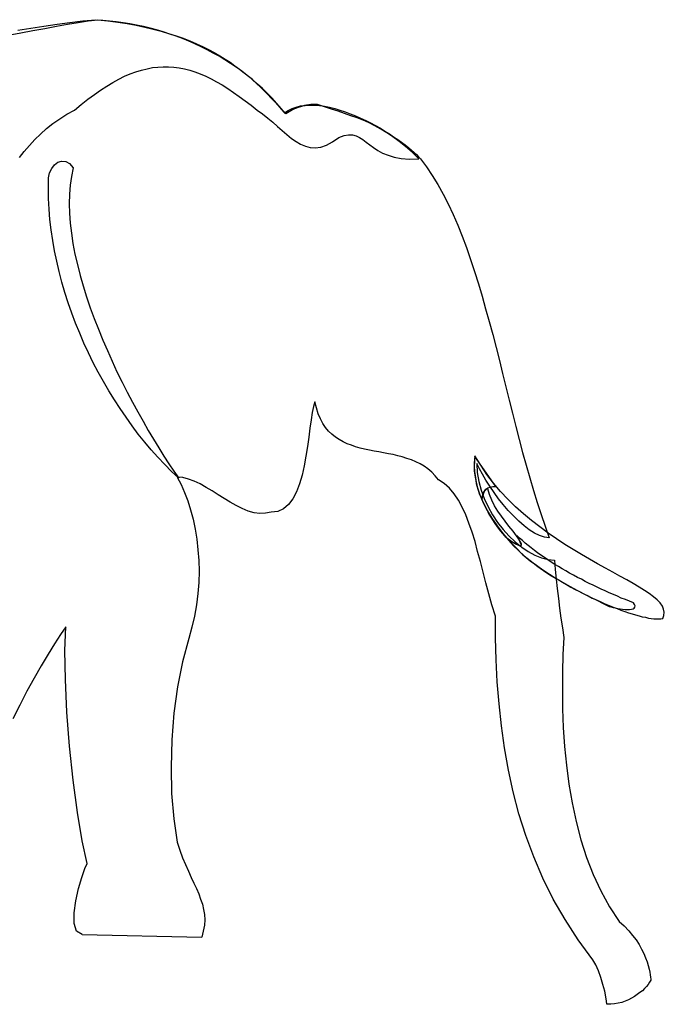
# Model space of a CAD drawing. Units: inches. Extents: x 386 to 107067, y -7 to 96314.
# Tile 8 of 10: x 101863.94 to 101865.933, y 96247.289 to 96250.334. Entities that reach past the tile are written whole.
import ezdxf

# ---------------------------------------------------------------- set-up
doc = ezdxf.new("R2010")
doc.units = ezdxf.units.IN
doc.layers.add('A-ELEV', color=7, linetype='Continuous', lineweight=25)
doc.layers.add('freecads.com', color=7, linetype='Continuous')

# ---------------------------------------------------------------- blocks, each defined once
blk = doc.blocks.new('elephant')
at = {"layer": 'freecads.com'}
for p, q in [((104458.6453, 95264.9047), (104458.6048, 95264.8987)), ((104458.6858, 95264.9107), (104458.6453, 95264.9047)), ((104458.6486, 95264.8987), (104458.6841, 95264.9052)), ((104458.6841, 95264.9052), (104458.7181, 95264.9113)), ((104458.7257, 95264.9162), (104458.6858, 95264.9107)), ((104458.7181, 95264.9113), (104458.7509, 95264.9167)), ((104458.7656, 95264.9206), (104458.7257, 95264.9162)), ((104458.7509, 95264.9167), (104458.782, 95264.9217)), ((104458.8055, 95264.9244), (104458.7656, 95264.9206)), ((104458.782, 95264.9217), (104458.8116, 95264.9255)), ((104458.8269, 95264.9227), (104458.8055, 95264.9244)), ((104458.8116, 95264.9255), (104458.8427, 95264.9222)), ((104458.8482, 95264.9211), (104458.8269, 95264.9227)), ((104458.8427, 95264.9222), (104458.8734, 95264.9178)), ((104458.869, 95264.9189), (104458.8482, 95264.9211)), ((104458.8903, 95264.9156), (104458.869, 95264.9189)), ((104458.8734, 95264.9178), (104458.9023, 95264.9134)), ((104458.9111, 95264.9124), (104458.8903, 95264.9156)), ((104458.9023, 95264.9134), (104458.9302, 95264.9085)), ((104458.9319, 95264.9085), (104458.9111, 95264.9124)), ((104458.9302, 95264.9085), (104458.957, 95264.9025)), ((104458.9527, 95264.9041), (104458.9319, 95264.9085)), ((104458.9734, 95264.8992), (104458.9527, 95264.9041)), ((104458.957, 95264.9025), (104458.9827, 95264.8965)), ((104458.5348, 95264.8773), (104458.5737, 95264.885)), ((104458.6048, 95264.8987), (104458.5644, 95264.8921)), ((104458.5737, 95264.885), (104458.6114, 95264.8921)), ((104458.6114, 95264.8921), (104458.6486, 95264.8987)), ((104458.9937, 95264.8938), (104458.9734, 95264.8992)), ((104458.9827, 95264.8965), (104459.0073, 95264.8899)), ((104459.0139, 95264.8877), (104458.9937, 95264.8938)), ((104459.0073, 95264.8899), (104459.0308, 95264.8828)), ((104459.0341, 95264.8812), (104459.0139, 95264.8877)), ((104459.0308, 95264.8828), (104459.0538, 95264.8757)), ((104459.0538, 95264.8741), (104459.0341, 95264.8812)), ((104459.0538, 95264.8757), (104459.0757, 95264.8681)), ((104459.0735, 95264.867), (104459.0538, 95264.8741)), ((104459.0932, 95264.8588), (104459.0735, 95264.867)), ((104459.0757, 95264.8681), (104459.0965, 95264.8599)), ((104459.1123, 95264.8506), (104459.0932, 95264.8588)), ((104459.0965, 95264.8599), (104459.1167, 95264.8511)), ((104459.1315, 95264.8418), (104459.1123, 95264.8506)), ((104459.1167, 95264.8511), (104459.1359, 95264.8424)), ((104459.1501, 95264.832), (104459.1315, 95264.8418)), ((104459.1359, 95264.8424), (104459.1544, 95264.8331)), ((104459.1687, 95264.8221), (104459.1501, 95264.832)), ((104459.1544, 95264.8331), (104459.1719, 95264.8238)), ((104459.1867, 95264.8123), (104459.1687, 95264.8221)), ((104459.1719, 95264.8238), (104459.1889, 95264.8139)), ((104459.2048, 95264.8013), (104459.1867, 95264.8123)), ((104459.1889, 95264.8139), (104459.2053, 95264.8035)), ((104458.9811, 95264.7773), (104458.9975, 95264.7789)), ((104458.9975, 95264.7789), (104459.0139, 95264.78)), ((104459.0139, 95264.78), (104459.0303, 95264.78)), ((104459.0303, 95264.78), (104459.0467, 95264.7789)), ((104459.0467, 95264.7789), (104459.0631, 95264.7767)), ((104459.2223, 95264.7899), (104459.2048, 95264.8013)), ((104459.2053, 95264.8035), (104459.2212, 95264.7937)), ((104459.2212, 95264.7937), (104459.2359, 95264.7833)), ((104459.2398, 95264.7784), (104459.2223, 95264.7899)), ((104459.2359, 95264.7833), (104459.2502, 95264.7724)), ((104458.8766, 95264.7412), (104458.8947, 95264.7505)), ((104458.8947, 95264.7505), (104458.9122, 95264.7581)), ((104458.9122, 95264.7581), (104458.9297, 95264.7642)), ((104458.9297, 95264.7642), (104458.9472, 95264.7696)), ((104458.9472, 95264.7696), (104458.9641, 95264.774)), ((104458.9641, 95264.774), (104458.9811, 95264.7773)), ((104459.0631, 95264.7767), (104459.0795, 95264.7735)), ((104459.0795, 95264.7735), (104459.0959, 95264.7691)), ((104459.0959, 95264.7691), (104459.1123, 95264.7642)), ((104459.1123, 95264.7642), (104459.1288, 95264.7576)), ((104459.1288, 95264.7576), (104459.1457, 95264.7505)), ((104459.1457, 95264.7505), (104459.1621, 95264.7423)), ((104459.2567, 95264.7658), (104459.2398, 95264.7784)), ((104459.2502, 95264.7724), (104459.2644, 95264.7614)), ((104459.2737, 95264.7532), (104459.2567, 95264.7658)), ((104459.2644, 95264.7614), (104459.2775, 95264.7505)), ((104459.2901, 95264.7401), (104459.2737, 95264.7532)), ((104459.2775, 95264.7505), (104459.2906, 95264.7395)), ((104458.8203, 95264.7078), (104458.8395, 95264.7204)), ((104458.8395, 95264.7204), (104458.8581, 95264.7313)), ((104458.8581, 95264.7313), (104458.8766, 95264.7412)), ((104459.1621, 95264.7423), (104459.179, 95264.7335)), ((104459.179, 95264.7335), (104459.196, 95264.7237)), ((104459.196, 95264.7237), (104459.2135, 95264.7128)), ((104459.3059, 95264.7264), (104459.2901, 95264.7401)), ((104459.2906, 95264.7395), (104459.3026, 95264.7281)), ((104459.3026, 95264.7281), (104459.3147, 95264.7171)), ((104459.3212, 95264.7122), (104459.3059, 95264.7264)), ((104458.7809, 95264.6794), (104458.8012, 95264.6942)), ((104458.8012, 95264.6942), (104458.8203, 95264.7078)), ((104459.2135, 95264.7128), (104459.231, 95264.7007)), ((104459.231, 95264.7007), (104459.2491, 95264.6882)), ((104459.2491, 95264.6882), (104459.2671, 95264.675)), ((104459.3147, 95264.7171), (104459.3262, 95264.7056)), ((104459.3366, 95264.6974), (104459.3212, 95264.7122)), ((104459.3262, 95264.7056), (104459.3376, 95264.6942)), ((104459.3513, 95264.6827), (104459.3366, 95264.6974)), ((104459.3376, 95264.6942), (104459.348, 95264.6827)), ((104458.7399, 95264.6455), (104458.7607, 95264.663)), ((104458.7607, 95264.663), (104458.7809, 95264.6794)), ((104459.2671, 95264.675), (104459.2857, 95264.6608)), ((104459.2857, 95264.6608), (104459.3043, 95264.6455)), ((104459.348, 95264.6827), (104459.359, 95264.6712)), ((104459.3655, 95264.6668), (104459.3513, 95264.6827)), ((104459.359, 95264.6712), (104459.3694, 95264.6597)), ((104459.3792, 95264.651), (104459.3655, 95264.6668)), ((104459.3694, 95264.6597), (104459.3792, 95264.6488)), ((104459.4251, 95264.6553), (104459.4383, 95264.6586)), ((104459.4383, 95264.6586), (104459.4525, 95264.6603)), ((104459.4443, 95264.6581), (104459.4383, 95264.6564)), ((104459.4508, 95264.6597), (104459.4443, 95264.6581)), ((104459.4574, 95264.6613), (104459.4508, 95264.6597)), ((104459.4525, 95264.6603), (104459.4667, 95264.6613)), ((104459.464, 95264.6624), (104459.4574, 95264.6613)), ((104459.4705, 95264.663), (104459.464, 95264.6624)), ((104459.4667, 95264.6613), (104459.4815, 95264.6613)), ((104459.4771, 95264.6635), (104459.4705, 95264.663)), ((104459.4842, 95264.6635), (104459.4771, 95264.6635)), ((104459.4815, 95264.6613), (104459.4968, 95264.6603)), ((104459.4908, 95264.663), (104459.4842, 95264.6635)), ((104459.5132, 95264.6559), (104459.4908, 95264.663)), ((104459.4968, 95264.6603), (104459.5127, 95264.6581)), ((104459.5127, 95264.6581), (104459.528, 95264.6548)), ((104458.6945, 95264.6192), (104458.7164, 95264.6329)), ((104458.7164, 95264.6329), (104458.7399, 95264.6455)), ((104459.3043, 95264.6455), (104459.3212, 95264.634)), ((104459.3212, 95264.634), (104459.3371, 95264.6214)), ((104459.3929, 95264.6345), (104459.3792, 95264.651)), ((104459.3792, 95264.6488), (104459.3891, 95264.6373)), ((104459.3891, 95264.6373), (104459.4005, 95264.6444)), ((104459.3978, 95264.6378), (104459.3929, 95264.6345)), ((104459.4033, 95264.6406), (104459.3978, 95264.6378)), ((104459.4005, 95264.6444), (104459.4126, 95264.6504)), ((104459.4087, 95264.6433), (104459.4033, 95264.6406)), ((104459.4142, 95264.6466), (104459.4087, 95264.6433)), ((104459.4126, 95264.6504), (104459.4251, 95264.6553)), ((104459.4197, 95264.6493), (104459.4142, 95264.6466)), ((104459.4257, 95264.6515), (104459.4197, 95264.6493)), ((104459.4317, 95264.6542), (104459.4257, 95264.6515)), ((104459.4383, 95264.6564), (104459.4317, 95264.6542)), ((104459.5345, 95264.6488), (104459.5132, 95264.6559)), ((104459.528, 95264.6548), (104459.5444, 95264.651)), ((104459.5553, 95264.6422), (104459.5345, 95264.6488)), ((104459.5444, 95264.651), (104459.5602, 95264.646)), ((104459.575, 95264.6356), (104459.5553, 95264.6422)), ((104459.5602, 95264.646), (104459.5761, 95264.6406)), ((104459.5941, 95264.6285), (104459.575, 95264.6356)), ((104459.5761, 95264.6406), (104459.5925, 95264.6345)), ((104459.5925, 95264.6345), (104459.6083, 95264.6285)), ((104459.6133, 95264.622), (104459.5941, 95264.6285)), ((104459.6083, 95264.6285), (104459.6242, 95264.6214)), ((104458.6535, 95264.5886), (104458.6732, 95264.6045)), ((104458.6732, 95264.6045), (104458.6945, 95264.6192)), ((104459.3371, 95264.6214), (104459.353, 95264.6083)), ((104459.353, 95264.6083), (104459.3677, 95264.5952)), ((104459.6319, 95264.6143), (104459.6133, 95264.622)), ((104459.6242, 95264.6214), (104459.6401, 95264.6138)), ((104459.6505, 95264.6061), (104459.6319, 95264.6143)), ((104459.6401, 95264.6138), (104459.6554, 95264.6061)), ((104459.6685, 95264.5974), (104459.6505, 95264.6061)), ((104459.6554, 95264.6061), (104459.6707, 95264.5979)), ((104459.6865, 95264.587), (104459.6685, 95264.5974)), ((104459.6707, 95264.5979), (104459.6855, 95264.5897)), ((104458.6174, 95264.5547), (104458.6349, 95264.5717)), ((104458.6349, 95264.5717), (104458.6535, 95264.5886)), ((104459.3677, 95264.5952), (104459.382, 95264.5826)), ((104459.382, 95264.5826), (104459.3962, 95264.57)), ((104459.3962, 95264.57), (104459.4104, 95264.5585)), ((104459.5575, 95264.5613), (104459.5733, 95264.5673)), ((104459.5733, 95264.5673), (104459.587, 95264.5695)), ((104459.587, 95264.5695), (104459.5996, 95264.5689)), ((104459.5996, 95264.5689), (104459.6105, 95264.5662)), ((104459.6105, 95264.5662), (104459.6209, 95264.5613)), ((104459.6855, 95264.5897), (104459.6997, 95264.581)), ((104459.7051, 95264.576), (104459.6865, 95264.587)), ((104459.6997, 95264.581), (104459.7133, 95264.5722)), ((104459.7243, 95264.5629), (104459.7051, 95264.576)), ((104459.7133, 95264.5722), (104459.7265, 95264.5635)), ((104458.5846, 95264.5181), (104458.6005, 95264.5367)), ((104458.6005, 95264.5367), (104458.6174, 95264.5547)), ((104459.4104, 95264.5585), (104459.4246, 95264.5487)), ((104459.4246, 95264.5487), (104459.4388, 95264.5405)), ((104459.4388, 95264.5405), (104459.4536, 95264.5345)), ((104459.5012, 95264.5317), (104459.5187, 95264.5378)), ((104459.5187, 95264.5378), (104459.5373, 95264.5476)), ((104459.5373, 95264.5476), (104459.5575, 95264.5613)), ((104459.6209, 95264.5613), (104459.6313, 95264.5547)), ((104459.6313, 95264.5547), (104459.6417, 95264.5471)), ((104459.6417, 95264.5471), (104459.6526, 95264.5389)), ((104459.6526, 95264.5389), (104459.6641, 95264.5301)), ((104459.7434, 95264.5487), (104459.7243, 95264.5629)), ((104459.7265, 95264.5635), (104459.739, 95264.5553)), ((104459.739, 95264.5553), (104459.7511, 95264.5465)), ((104459.7631, 95264.5328), (104459.7434, 95264.5487)), ((104459.7511, 95264.5465), (104459.762, 95264.5383)), ((104459.762, 95264.5383), (104459.7724, 95264.5301)), ((104458.5693, 95264.4995), (104458.5846, 95264.5181)), ((104459.4536, 95264.5345), (104459.4683, 95264.5306)), ((104459.4683, 95264.5306), (104459.4842, 95264.5296)), ((104459.4842, 95264.5296), (104459.5012, 95264.5317)), ((104459.6641, 95264.5301), (104459.6773, 95264.5213)), ((104459.6773, 95264.5213), (104459.692, 95264.5131)), ((104459.692, 95264.5131), (104459.709, 95264.506)), ((104459.709, 95264.506), (104459.7281, 95264.5)), ((104459.7833, 95264.5153), (104459.7631, 95264.5328)), ((104459.7724, 95264.5301), (104459.7817, 95264.5224)), ((104459.7817, 95264.5224), (104459.7899, 95264.5148)), ((104459.8047, 95264.4951), (104459.7833, 95264.5153)), ((104459.7899, 95264.5148), (104459.7976, 95264.5082)), ((104459.7976, 95264.5082), (104459.8036, 95264.5017)), ((104458.6694, 95264.4656), (104458.6781, 95264.4765)), ((104458.6781, 95264.4765), (104458.6885, 95264.4847)), ((104458.6885, 95264.4847), (104458.7, 95264.488)), ((104458.7, 95264.488), (104458.7126, 95264.4869)), ((104458.7126, 95264.4869), (104458.7246, 95264.4803)), ((104458.7246, 95264.4803), (104458.7361, 95264.4672)), ((104459.7281, 95264.5), (104459.75, 95264.4962)), ((104459.75, 95264.4962), (104459.7757, 95264.4945)), ((104459.7757, 95264.4945), (104459.8047, 95264.4951)), ((104459.8036, 95264.5017), (104459.809, 95264.4956)), ((104459.809, 95264.4956), (104459.8276, 95264.4705)), ((104458.6595, 95264.436), (104458.6628, 95264.4519)), ((104458.6628, 95264.4519), (104458.6694, 95264.4656)), ((104458.7361, 95264.4672), (104458.7301, 95264.441)), ((104459.8276, 95264.4705), (104459.8457, 95264.4437)), ((104459.8457, 95264.4437), (104459.8632, 95264.4158)), ((104458.659, 95264.4043), (104458.6595, 95264.436)), ((104458.7263, 95264.4136), (104458.7241, 95264.3857)), ((104458.7301, 95264.441), (104458.7263, 95264.4136)), ((104459.8632, 95264.4158), (104459.8796, 95264.3863)), ((104458.6595, 95264.3721), (104458.659, 95264.4043)), ((104458.7241, 95264.3857), (104458.723, 95264.3562)), ((104459.8796, 95264.3863), (104459.8949, 95264.3556)), ((104458.6612, 95264.3398), (104458.6595, 95264.3721)), ((104458.723, 95264.3562), (104458.7241, 95264.3267)), ((104459.8949, 95264.3556), (104459.9102, 95264.3234)), ((104458.6639, 95264.3075), (104458.6612, 95264.3398)), ((104458.7241, 95264.3267), (104458.7263, 95264.296)), ((104459.9102, 95264.3234), (104459.9244, 95264.29)), ((104458.6677, 95264.2753), (104458.6639, 95264.3075)), ((104458.7263, 95264.296), (104458.7301, 95264.2649)), ((104458.6727, 95264.243), (104458.6677, 95264.2753)), ((104458.7301, 95264.2649), (104458.735, 95264.2331)), ((104459.9244, 95264.29), (104459.9381, 95264.2556)), ((104458.6781, 95264.2107), (104458.6727, 95264.243)), ((104458.735, 95264.2331), (104458.741, 95264.2003)), ((104459.9381, 95264.2556), (104459.9512, 95264.2206)), ((104458.6847, 95264.1785), (104458.6781, 95264.2107)), ((104458.741, 95264.2003), (104458.7487, 95264.1681)), ((104459.9512, 95264.2206), (104459.9643, 95264.1839)), ((104458.6924, 95264.1462), (104458.6847, 95264.1785)), ((104459.9643, 95264.1839), (104459.9764, 95264.1468)), ((104458.7011, 95264.1139), (104458.6924, 95264.1462)), ((104458.7487, 95264.1681), (104458.7569, 95264.1347)), ((104459.9764, 95264.1468), (104459.9884, 95264.109)), ((104458.7104, 95264.0817), (104458.7011, 95264.1139)), ((104458.7569, 95264.1347), (104458.7667, 95264.1019)), ((104459.9884, 95264.109), (104459.9999, 95264.0707)), ((104458.7202, 95264.0499), (104458.7104, 95264.0817)), ((104458.7667, 95264.1019), (104458.7771, 95264.0685)), ((104458.7312, 95264.0182), (104458.7202, 95264.0499)), ((104458.7771, 95264.0685), (104458.7886, 95264.0346)), ((104459.9999, 95264.0707), (104460.0108, 95264.0314)), ((104458.7432, 95263.9871), (104458.7312, 95264.0182)), ((104458.7886, 95264.0346), (104458.8006, 95264.0013)), ((104460.0108, 95264.0314), (104460.0218, 95263.992)), ((104458.7558, 95263.9559), (104458.7432, 95263.9871)), ((104458.8006, 95264.0013), (104458.8138, 95263.9679)), ((104460.0218, 95263.992), (104460.0327, 95263.9521)), ((104458.8138, 95263.9679), (104458.8274, 95263.9346)), ((104458.7689, 95263.9253), (104458.7558, 95263.9559)), ((104458.8274, 95263.9346), (104458.8416, 95263.9018)), ((104460.0327, 95263.9521), (104460.0431, 95263.9116)), ((104458.7831, 95263.8946), (104458.7689, 95263.9253)), ((104458.8416, 95263.9018), (104458.8559, 95263.8689)), ((104460.0431, 95263.9116), (104460.0535, 95263.8711)), ((104458.7973, 95263.8646), (104458.7831, 95263.8946)), ((104458.8559, 95263.8689), (104458.8712, 95263.8367)), ((104460.0535, 95263.8711), (104460.0633, 95263.8307)), ((104458.8132, 95263.835), (104458.7973, 95263.8646)), ((104458.8291, 95263.806), (104458.8132, 95263.835)), ((104458.8712, 95263.8367), (104458.887, 95263.8044)), ((104458.8455, 95263.7776), (104458.8291, 95263.806)), ((104458.887, 95263.8044), (104458.9029, 95263.7732)), ((104460.0633, 95263.8307), (104460.0737, 95263.7896)), ((104458.863, 95263.7497), (104458.8455, 95263.7776)), ((104460.0737, 95263.7896), (104460.0841, 95263.7486)), ((104458.8805, 95263.7224), (104458.863, 95263.7497)), ((104458.9029, 95263.7732), (104458.9187, 95263.7426)), ((104459.4831, 95263.7437), (104459.4787, 95263.7289)), ((104459.4875, 95263.7246), (104459.4831, 95263.7437)), ((104460.0841, 95263.7486), (104460.094, 95263.7082)), ((104458.8991, 95263.6956), (104458.8805, 95263.7224)), ((104458.9187, 95263.7426), (104458.9352, 95263.7125)), ((104459.4787, 95263.7289), (104459.4749, 95263.7103)), ((104459.4935, 95263.7065), (104459.4875, 95263.7246)), ((104458.9176, 95263.6694), (104458.8991, 95263.6956)), ((104458.9352, 95263.7125), (104458.9516, 95263.6835)), ((104458.9516, 95263.6835), (104458.968, 95263.6551)), ((104459.4711, 95263.6874), (104459.4678, 95263.6622)), ((104459.4749, 95263.7103), (104459.4711, 95263.6874)), ((104459.5001, 95263.6912), (104459.4935, 95263.7065)), ((104459.5077, 95263.677), (104459.5001, 95263.6912)), ((104460.094, 95263.7082), (104460.1043, 95263.6677)), ((104458.9368, 95263.6436), (104458.9176, 95263.6694)), ((104458.968, 95263.6551), (104458.9838, 95263.6278)), ((104459.4678, 95263.6622), (104459.464, 95263.6343)), ((104459.5159, 95263.6639), (104459.5077, 95263.677)), ((104459.5252, 95263.6529), (104459.5159, 95263.6639)), ((104459.5356, 95263.6431), (104459.5252, 95263.6529)), ((104460.1043, 95263.6677), (104460.1147, 95263.6272)), ((104458.957, 95263.619), (104458.9368, 95263.6436)), ((104458.9838, 95263.6278), (104459.0002, 95263.601)), ((104459.464, 95263.6343), (104459.4601, 95263.6054)), ((104459.5466, 95263.6343), (104459.5356, 95263.6431)), ((104459.558, 95263.6267), (104459.5466, 95263.6343)), ((104459.5701, 95263.6196), (104459.558, 95263.6267)), ((104460.1147, 95263.6272), (104460.1251, 95263.5873)), ((104458.9773, 95263.595), (104458.957, 95263.619)), ((104458.9975, 95263.572), (104458.9773, 95263.595)), ((104459.0002, 95263.601), (104459.0161, 95263.5758)), ((104459.4601, 95263.6054), (104459.4552, 95263.5753)), ((104459.5826, 95263.6141), (104459.5701, 95263.6196)), ((104459.5958, 95263.6092), (104459.5826, 95263.6141)), ((104459.6089, 95263.6043), (104459.5958, 95263.6092)), ((104459.6226, 95263.6004), (104459.6089, 95263.6043)), ((104459.6368, 95263.5972), (104459.6226, 95263.6004)), ((104459.6516, 95263.5944), (104459.6368, 95263.5972)), ((104459.6658, 95263.5912), (104459.6516, 95263.5944)), ((104459.6805, 95263.5884), (104459.6658, 95263.5912)), ((104459.0188, 95263.5496), (104458.9975, 95263.572)), ((104459.0161, 95263.5758), (104459.0319, 95263.5518)), ((104459.4552, 95263.5753), (104459.4497, 95263.5458)), ((104459.6953, 95263.5857), (104459.6805, 95263.5884)), ((104459.7101, 95263.583), (104459.6953, 95263.5857)), ((104459.7248, 95263.5802), (104459.7101, 95263.583)), ((104459.739, 95263.5769), (104459.7248, 95263.5802)), ((104459.7533, 95263.5731), (104459.739, 95263.5769)), ((104459.7675, 95263.5687), (104459.7533, 95263.5731)), ((104459.7817, 95263.5638), (104459.7675, 95263.5687)), ((104459.7948, 95263.5583), (104459.7817, 95263.5638)), ((104459.9775, 95263.5769), (104459.9753, 95263.5534)), ((104459.9764, 95263.5605), (104459.9758, 95263.5447)), ((104459.9775, 95263.5748), (104459.9764, 95263.5605)), ((104459.9955, 95263.5474), (104459.9775, 95263.5769)), ((104460.042, 95263.4812), (104459.9775, 95263.5748)), ((104460.1251, 95263.5873), (104460.1361, 95263.5474)), ((104459.0401, 95263.5283), (104459.0188, 95263.5496)), ((104459.0319, 95263.5518), (104459.0473, 95263.5288)), ((104459.4497, 95263.5458), (104459.4432, 95263.5168)), ((104459.808, 95263.5518), (104459.7948, 95263.5583)), ((104459.8205, 95263.5441), (104459.808, 95263.5518)), ((104459.8326, 95263.5359), (104459.8205, 95263.5441)), ((104459.8446, 95263.5261), (104459.8326, 95263.5359)), ((104459.9753, 95263.5534), (104459.9758, 95263.5294)), ((104459.9758, 95263.5447), (104459.9769, 95263.5272)), ((104459.9917, 95263.5365), (104459.9835, 95263.5523)), ((104459.9835, 95263.5523), (104459.9851, 95263.525)), ((104460.001, 95263.5195), (104459.9917, 95263.5365)), ((104460.0147, 95263.519), (104459.9955, 95263.5474)), ((104460.1361, 95263.5474), (104460.147, 95263.5086)), ((104459.062, 95263.5075), (104459.0401, 95263.5283)), ((104459.0473, 95263.5288), (104459.062, 95263.5075)), ((104459.0746, 95263.5091), (104459.0576, 95263.5108)), ((104459.0576, 95263.5108), (104459.0691, 95263.4878)), ((104459.0921, 95263.5047), (104459.0746, 95263.5091)), ((104459.1102, 95263.4982), (104459.0921, 95263.5047)), ((104459.4432, 95263.5168), (104459.4355, 95263.49)), ((104459.855, 95263.5151), (104459.8446, 95263.5261)), ((104459.8654, 95263.5026), (104459.855, 95263.5151)), ((104459.8829, 95263.4911), (104459.8654, 95263.5026)), ((104459.9758, 95263.5294), (104459.9791, 95263.5053)), ((104459.9769, 95263.5272), (104459.9791, 95263.5091)), ((104459.9791, 95263.5091), (104459.9818, 95263.4911)), ((104459.9791, 95263.5053), (104459.9851, 95263.4807)), ((104459.9851, 95263.525), (104459.9895, 95263.4976)), ((104460.0119, 95263.5009), (104460.001, 95263.5195)), ((104460.024, 95263.4823), (104460.0119, 95263.5009)), ((104460.0349, 95263.4922), (104460.0147, 95263.519)), ((104460.147, 95263.5086), (104460.1585, 95263.4697)), ((104459.0691, 95263.4878), (104459.0801, 95263.4632)), ((104459.1282, 95263.4894), (104459.1102, 95263.4982)), ((104459.1468, 95263.479), (104459.1282, 95263.4894)), ((104459.1654, 95263.4681), (104459.1468, 95263.479)), ((104459.4355, 95263.49), (104459.4257, 95263.4648)), ((104459.8987, 95263.4763), (104459.8829, 95263.4911)), ((104459.9135, 95263.4594), (104459.8987, 95263.4763)), ((104459.9818, 95263.4911), (104459.9868, 95263.4736)), ((104459.9851, 95263.4807), (104459.9933, 95263.4561)), ((104459.9868, 95263.4736), (104459.9922, 95263.4572)), ((104459.9895, 95263.4976), (104459.9966, 95263.4708)), ((104459.9966, 95263.4708), (104460.0065, 95263.4446)), ((104460.007, 95263.4676), (104460.0119, 95263.4736)), ((104460.0103, 95263.4703), (104460.0076, 95263.467)), ((104460.0136, 95263.473), (104460.0103, 95263.4703)), ((104460.0119, 95263.4736), (104460.0179, 95263.4774)), ((104460.0174, 95263.4747), (104460.0136, 95263.473)), ((104460.0229, 95263.4566), (104460.0174, 95263.4747)), ((104460.0179, 95263.4774), (104460.0245, 95263.4801)), ((104460.0371, 95263.4632), (104460.024, 95263.4823)), ((104460.0245, 95263.4801), (104460.0327, 95263.4812)), ((104460.0327, 95263.4812), (104460.042, 95263.4812)), ((104460.0568, 95263.4665), (104460.0349, 95263.4922)), ((104460.1585, 95263.4697), (104460.17, 95263.432)), ((104459.0801, 95263.4632), (104459.0899, 95263.4369)), ((104459.184, 95263.4561), (104459.1654, 95263.4681)), ((104459.2026, 95263.4446), (104459.184, 95263.4561)), ((104459.2212, 95263.4331), (104459.2026, 95263.4446)), ((104459.4148, 95263.4435), (104459.4016, 95263.4255)), ((104459.4257, 95263.4648), (104459.4148, 95263.4435)), ((104459.9266, 95263.4397), (104459.9135, 95263.4594)), ((104459.9387, 95263.4178), (104459.9266, 95263.4397)), ((104459.9922, 95263.4572), (104459.9999, 95263.4424)), ((104459.9933, 95263.4561), (104460.0037, 95263.4315)), ((104460.0004, 95263.4473), (104459.9988, 95263.4419)), ((104459.9988, 95263.4419), (104460.0065, 95263.4255)), ((104459.9999, 95263.4424), (104460.001, 95263.4522)), ((104460.0021, 95263.4528), (104460.0004, 95263.4473)), ((104460.001, 95263.4522), (104460.0037, 95263.461)), ((104460.0032, 95263.4577), (104460.0021, 95263.4528)), ((104460.0054, 95263.4626), (104460.0032, 95263.4577)), ((104460.0037, 95263.461), (104460.007, 95263.4676)), ((104460.0076, 95263.467), (104460.0054, 95263.4626)), ((104460.0065, 95263.4446), (104460.0185, 95263.4189)), ((104460.03, 95263.4397), (104460.0229, 95263.4566)), ((104460.0387, 95263.4222), (104460.03, 95263.4397)), ((104460.0508, 95263.444), (104460.0371, 95263.4632)), ((104460.0655, 95263.4255), (104460.0508, 95263.444)), ((104460.0797, 95263.4424), (104460.0568, 95263.4665)), ((104460.1033, 95263.4189), (104460.0797, 95263.4424)), ((104459.0899, 95263.4369), (104459.0987, 95263.4091)), ((104459.0987, 95263.4091), (104459.1063, 95263.3801)), ((104459.2398, 95263.4227), (104459.2212, 95263.4331)), ((104459.2584, 95263.4134), (104459.2398, 95263.4227)), ((104459.2769, 95263.4058), (104459.2584, 95263.4134)), ((104459.3858, 95263.4123), (104459.3683, 95263.4041)), ((104459.4016, 95263.4255), (104459.3858, 95263.4123)), ((104459.9496, 95263.3937), (104459.9387, 95263.4178)), ((104460.0037, 95263.4315), (104460.0158, 95263.4074)), ((104460.0065, 95263.4255), (104460.0141, 95263.4101)), ((104460.0141, 95263.4101), (104460.0212, 95263.3965)), ((104460.0185, 95263.4189), (104460.0322, 95263.3943)), ((104460.0486, 95263.4058), (104460.0387, 95263.4222)), ((104460.0808, 95263.4074), (104460.0655, 95263.4255)), ((104460.1279, 95263.397), (104460.1033, 95263.4189)), ((104460.17, 95263.432), (104460.182, 95263.3948)), ((104459.1063, 95263.3801), (104459.1129, 95263.3494)), ((104459.295, 95263.4003), (104459.2769, 95263.4058)), ((104459.313, 95263.3981), (104459.295, 95263.4003)), ((104459.3305, 95263.3987), (104459.313, 95263.3981)), ((104459.3475, 95263.4025), (104459.3305, 95263.3987)), ((104459.3683, 95263.4041), (104459.3475, 95263.4025)), ((104459.9594, 95263.368), (104459.9496, 95263.3937)), ((104460.0158, 95263.4074), (104460.03, 95263.3833)), ((104460.0212, 95263.3965), (104460.0289, 95263.3833)), ((104460.0289, 95263.3833), (104460.0371, 95263.3702)), ((104460.03, 95263.3833), (104460.0464, 95263.3598)), ((104460.0322, 95263.3943), (104460.048, 95263.3708)), ((104460.0595, 95263.3899), (104460.0486, 95263.4058)), ((104460.071, 95263.374), (104460.0595, 95263.3899)), ((104460.0967, 95263.3905), (104460.0808, 95263.4074)), ((104460.1131, 95263.3746), (104460.0967, 95263.3905)), ((104460.1525, 95263.3762), (104460.1279, 95263.397)), ((104460.182, 95263.3948), (104460.1946, 95263.3587)), ((104459.1129, 95263.3494), (104459.1178, 95263.3183)), ((104459.9687, 95263.3407), (104459.9594, 95263.368)), ((104460.0371, 95263.3702), (104460.0464, 95263.3571)), ((104460.0464, 95263.3598), (104460.0639, 95263.3363)), ((104460.0464, 95263.3571), (104460.0568, 95263.3434)), ((104460.048, 95263.3708), (104460.065, 95263.3489)), ((104460.065, 95263.3489), (104460.083, 95263.3287)), ((104460.083, 95263.3587), (104460.071, 95263.374)), ((104460.0956, 95263.344), (104460.083, 95263.3587)), ((104460.1295, 95263.3598), (104460.1131, 95263.3746)), ((104460.1454, 95263.3478), (104460.1295, 95263.3598)), ((104460.1618, 95263.3374), (104460.1454, 95263.3478)), ((104460.1782, 95263.3565), (104460.1525, 95263.3762)), ((104460.2039, 95263.3374), (104460.1782, 95263.3565)), ((104460.1946, 95263.3587), (104460.2077, 95263.3232)), ((104459.1178, 95263.3183), (104459.1216, 95263.286)), ((104459.978, 95263.3117), (104459.9687, 95263.3407)), ((104460.0568, 95263.3434), (104460.0688, 95263.3287)), ((104460.0639, 95263.3363), (104460.083, 95263.3144)), ((104460.0688, 95263.3287), (104460.0715, 95263.3265)), ((104460.0715, 95263.3265), (104460.0754, 95263.3237)), ((104460.0754, 95263.3237), (104460.0803, 95263.3199)), ((104460.0803, 95263.3199), (104460.0863, 95263.3155)), ((104460.083, 95263.3287), (104460.1022, 95263.3101)), ((104460.106, 95263.3292), (104460.0956, 95263.344)), ((104460.1136, 95263.3183), (104460.106, 95263.3292)), ((104460.1076, 95263.3297), (104460.1125, 95263.321)), ((104460.1158, 95263.3221), (104460.1076, 95263.3297)), ((104460.1125, 95263.321), (104460.1169, 95263.3128)), ((104460.118, 95263.3095), (104460.1136, 95263.3183)), ((104460.1246, 95263.3144), (104460.1158, 95263.3221)), ((104460.1776, 95263.3297), (104460.1618, 95263.3374)), ((104460.193, 95263.3248), (104460.1776, 95263.3297)), ((104460.2077, 95263.3232), (104460.193, 95263.3248)), ((104460.2301, 95263.3194), (104460.2039, 95263.3374)), ((104460.2558, 95263.3024), (104460.2301, 95263.3194)), ((104459.9862, 95263.2811), (104459.978, 95263.3117)), ((104460.1, 95263.3051), (104460.0814, 95263.3161)), ((104460.0814, 95263.3161), (104460.0961, 95263.2991)), ((104460.083, 95263.3144), (104460.1038, 95263.2926)), ((104460.0863, 95263.3155), (104460.0923, 95263.3112)), ((104460.0923, 95263.3112), (104460.0989, 95263.3073)), ((104460.0961, 95263.2991), (104460.1125, 95263.2833)), ((104460.0989, 95263.3073), (104460.1049, 95263.3035)), ((104460.112, 95263.2997), (104460.1, 95263.3051)), ((104460.1022, 95263.3101), (104460.1224, 95263.2942)), ((104460.1038, 95263.2926), (104460.1251, 95263.2718)), ((104460.1049, 95263.3035), (104460.1104, 95263.3008)), ((104460.1104, 95263.3008), (104460.1147, 95263.2991)), ((104460.1186, 95263.2986), (104460.112, 95263.2997)), ((104460.1147, 95263.2991), (104460.1186, 95263.2991)), ((104460.1169, 95263.3128), (104460.1202, 95263.3057)), ((104460.1202, 95263.3041), (104460.118, 95263.3095)), ((104460.1207, 95263.3008), (104460.1186, 95263.2986)), ((104460.1186, 95263.2991), (104460.1202, 95263.3002)), ((104460.1202, 95263.3057), (104460.1207, 95263.3008)), ((104460.1202, 95263.3002), (104460.1202, 95263.3041)), ((104460.1224, 95263.2942), (104460.1426, 95263.2805)), ((104460.1333, 95263.3068), (104460.1246, 95263.3144)), ((104460.1426, 95263.2991), (104460.1333, 95263.3068)), ((104460.1519, 95263.2915), (104460.1426, 95263.2991)), ((104460.1618, 95263.2838), (104460.1519, 95263.2915)), ((104460.2815, 95263.2866), (104460.2558, 95263.3024)), ((104460.3072, 95263.2712), (104460.2815, 95263.2866)), ((104459.1216, 95263.286), (104459.1238, 95263.2532)), ((104459.995, 95263.2499), (104459.9862, 95263.2811)), ((104460.1125, 95263.2833), (104460.13, 95263.2674)), ((104460.1251, 95263.2718), (104460.1481, 95263.2526)), ((104460.13, 95263.2674), (104460.1481, 95263.2521)), ((104460.1426, 95263.2805), (104460.1634, 95263.2696)), ((104460.1716, 95263.2767), (104460.1618, 95263.2838)), ((104460.1634, 95263.2696), (104460.1837, 95263.2614)), ((104460.1815, 95263.2691), (104460.1716, 95263.2767)), ((104460.1924, 95263.2619), (104460.1815, 95263.2691)), ((104460.1837, 95263.2614), (104460.2039, 95263.2559)), ((104460.2028, 95263.2548), (104460.1924, 95263.2619)), ((104460.2039, 95263.2559), (104460.2236, 95263.2543)), ((104460.3324, 95263.2565), (104460.3072, 95263.2712)), ((104460.357, 95263.2428), (104460.3324, 95263.2565)), ((104459.1238, 95263.2532), (104459.1249, 95263.2193)), ((104460.0032, 95263.2171), (104459.995, 95263.2499)), ((104460.1481, 95263.2526), (104460.1722, 95263.234)), ((104460.1481, 95263.2521), (104460.1678, 95263.2379)), ((104460.1678, 95263.2379), (104460.1875, 95263.2237)), ((104460.1722, 95263.234), (104460.1968, 95263.2171)), ((104460.2137, 95263.2477), (104460.2028, 95263.2548)), ((104460.2247, 95263.2406), (104460.2137, 95263.2477)), ((104460.2236, 95263.2543), (104460.2258, 95263.2247)), ((104460.2361, 95263.234), (104460.2247, 95263.2406)), ((104460.2476, 95263.2269), (104460.2361, 95263.234)), ((104460.2591, 95263.2204), (104460.2476, 95263.2269)), ((104460.3811, 95263.2291), (104460.357, 95263.2428)), ((104460.404, 95263.2165), (104460.3811, 95263.2291)), ((104459.1249, 95263.2193), (104459.1238, 95263.1848)), ((104460.0119, 95263.1837), (104460.0032, 95263.2171)), ((104460.1875, 95263.2237), (104460.2083, 95263.21)), ((104460.1968, 95263.2171), (104460.2094, 95263.2089)), ((104460.2083, 95263.21), (104460.229, 95263.1969)), ((104460.2094, 95263.2089), (104460.2219, 95263.2012)), ((104460.2219, 95263.2012), (104460.235, 95263.1936)), ((104460.2258, 95263.2247), (104460.229, 95263.1952)), ((104460.229, 95263.1969), (104460.2504, 95263.1843)), ((104460.229, 95263.1952), (104460.2323, 95263.1657)), ((104460.2706, 95263.2138), (104460.2591, 95263.2204)), ((104460.2826, 95263.2072), (104460.2706, 95263.2138)), ((104460.2947, 95263.2007), (104460.2826, 95263.2072)), ((104460.3067, 95263.1947), (104460.2947, 95263.2007)), ((104460.4259, 95263.2045), (104460.404, 95263.2165)), ((104460.4472, 95263.193), (104460.4259, 95263.2045)), ((104459.1238, 95263.1848), (104459.1216, 95263.1504)), ((104460.0212, 95263.1498), (104460.0119, 95263.1837)), ((104460.2323, 95263.1657), (104460.2356, 95263.1356)), ((104460.235, 95263.1936), (104460.2482, 95263.1854)), ((104460.2482, 95263.1854), (104460.2613, 95263.1783)), ((104460.2504, 95263.1843), (104460.2717, 95263.1723)), ((104460.2613, 95263.1783), (104460.2744, 95263.1706)), ((104460.2717, 95263.1723), (104460.293, 95263.1608)), ((104460.2744, 95263.1706), (104460.2875, 95263.1635)), ((104460.3187, 95263.1881), (104460.3067, 95263.1947)), ((104460.3313, 95263.1821), (104460.3187, 95263.1881)), ((104460.3433, 95263.1761), (104460.3313, 95263.1821)), ((104460.3559, 95263.1701), (104460.3433, 95263.1761)), ((104460.3679, 95263.1646), (104460.3559, 95263.1701)), ((104460.3805, 95263.1586), (104460.3679, 95263.1646)), ((104460.4669, 95263.1816), (104460.4472, 95263.193)), ((104460.485, 95263.1706), (104460.4669, 95263.1816)), ((104460.5019, 95263.1602), (104460.485, 95263.1706)), ((104459.1216, 95263.1504), (104459.1173, 95263.1159)), ((104460.0305, 95263.1154), (104460.0212, 95263.1498)), ((104460.2356, 95263.1356), (104460.2394, 95263.1055)), ((104460.2875, 95263.1635), (104460.3012, 95263.1564)), ((104460.293, 95263.1608), (104460.3144, 95263.1498)), ((104460.3012, 95263.1564), (104460.3144, 95263.1498)), ((104460.3144, 95263.1498), (104460.3346, 95263.1394)), ((104460.3144, 95263.1498), (104460.3275, 95263.1433)), ((104460.3275, 95263.1433), (104460.3406, 95263.1367)), ((104460.3346, 95263.1394), (104460.3548, 95263.1296)), ((104460.3406, 95263.1367), (104460.3537, 95263.1307)), ((104460.3931, 95263.1531), (104460.3805, 95263.1586)), ((104460.4057, 95263.1477), (104460.3931, 95263.1531)), ((104460.4182, 95263.1422), (104460.4057, 95263.1477)), ((104460.4303, 95263.1367), (104460.4182, 95263.1422)), ((104460.4429, 95263.1318), (104460.4303, 95263.1367)), ((104460.5167, 95263.1504), (104460.5019, 95263.1602)), ((104460.5298, 95263.1405), (104460.5167, 95263.1504)), ((104460.5413, 95263.1307), (104460.5298, 95263.1405)), ((104459.1173, 95263.1159), (104459.1113, 95263.0809)), ((104460.0409, 95263.0804), (104460.0305, 95263.1154)), ((104460.2394, 95263.1055), (104460.2438, 95263.0749)), ((104460.3537, 95263.1307), (104460.3668, 95263.1247)), ((104460.3548, 95263.1296), (104460.3745, 95263.1198)), ((104460.3668, 95263.1247), (104460.3794, 95263.1192)), ((104460.3745, 95263.1198), (104460.3931, 95263.111)), ((104460.3794, 95263.1192), (104460.3925, 95263.1137)), ((104460.3925, 95263.1137), (104460.4046, 95263.1088)), ((104460.3931, 95263.111), (104460.398, 95263.1094)), ((104460.398, 95263.1094), (104460.4046, 95263.1077)), ((104460.4046, 95263.1088), (104460.4172, 95263.1039)), ((104460.4046, 95263.1077), (104460.4111, 95263.1061)), ((104460.4111, 95263.1061), (104460.4188, 95263.1044)), ((104460.4172, 95263.1039), (104460.4292, 95263.099)), ((104460.4188, 95263.1044), (104460.4265, 95263.1028)), ((104460.4554, 95263.1269), (104460.4429, 95263.1318)), ((104460.4675, 95263.1219), (104460.4554, 95263.1269)), ((104460.4669, 95263.1033), (104460.4702, 95263.1055)), ((104460.4713, 95263.1165), (104460.4675, 95263.1219)), ((104460.4702, 95263.1055), (104460.4724, 95263.1083)), ((104460.4729, 95263.1121), (104460.4713, 95263.1165)), ((104460.4724, 95263.1083), (104460.4729, 95263.1121)), ((104460.55, 95263.1214), (104460.5413, 95263.1307)), ((104460.5572, 95263.1116), (104460.55, 95263.1214)), ((104460.561, 95263.1023), (104460.5572, 95263.1116)), ((104459.1113, 95263.0809), (104459.103, 95263.0465)), ((104460.0415, 95263.0131), (104460.0409, 95263.0804)), ((104460.2438, 95263.0749), (104460.2482, 95263.0448)), ((104460.4265, 95263.1028), (104460.4341, 95263.1023)), ((104460.4292, 95263.099), (104460.4407, 95263.0951)), ((104460.4341, 95263.1023), (104460.4423, 95263.1012)), ((104460.4407, 95263.0951), (104460.4522, 95263.0913)), ((104460.4423, 95263.1012), (104460.4494, 95263.1012)), ((104460.4494, 95263.1012), (104460.456, 95263.1012)), ((104460.4522, 95263.0913), (104460.4637, 95263.0875)), ((104460.456, 95263.1012), (104460.462, 95263.1023)), ((104460.462, 95263.1023), (104460.4669, 95263.1033)), ((104460.4637, 95263.0875), (104460.4746, 95263.0842)), ((104460.4746, 95263.0842), (104460.485, 95263.0815)), ((104460.485, 95263.0815), (104460.4948, 95263.0787)), ((104460.4948, 95263.0787), (104460.5047, 95263.0771)), ((104460.5047, 95263.0771), (104460.5139, 95263.0749)), ((104460.5139, 95263.0749), (104460.5227, 95263.0738)), ((104460.5227, 95263.0738), (104460.5309, 95263.0727)), ((104460.5522, 95263.0727), (104460.5582, 95263.0738)), ((104460.5582, 95263.0738), (104460.5621, 95263.0831)), ((104460.5632, 95263.093), (104460.561, 95263.1023)), ((104460.5621, 95263.0831), (104460.5632, 95263.093)), ((104458.7131, 95263.0481), (104458.6967, 95263.0241)), ((104458.7099, 95262.9748), (104458.7131, 95263.0481)), ((104459.103, 95263.0465), (104459.0932, 95263.012)), ((104460.2482, 95263.0448), (104460.2525, 95263.0142)), ((104460.5309, 95263.0727), (104460.5386, 95263.0727)), ((104460.5386, 95263.0727), (104460.5457, 95263.0727)), ((104460.5457, 95263.0727), (104460.5522, 95263.0727)), ((104458.6967, 95263.0241), (104458.6781, 95262.9951)), ((104460.0437, 95262.9453), (104460.0415, 95263.0131)), ((104460.2525, 95263.0142), (104460.2498, 95262.9617)), ((104458.6781, 95262.9951), (104458.6584, 95262.9628)), ((104459.0932, 95263.012), (104459.0735, 95262.9398)), ((104458.6584, 95262.9628), (104458.6371, 95262.9273)), ((104458.7115, 95262.8852), (104458.7099, 95262.9748)), ((104460.2498, 95262.9617), (104460.2487, 95262.907)), ((104458.6371, 95262.9273), (104458.6147, 95262.889)), ((104459.0735, 95262.9398), (104459.0582, 95262.8622)), ((104460.0469, 95262.8775), (104460.0437, 95262.9453)), ((104460.2487, 95262.907), (104460.2482, 95262.8512)), ((104458.6147, 95262.889), (104458.5928, 95262.8485)), ((104458.7164, 95262.784), (104458.7115, 95262.8852)), ((104459.0582, 95262.8622), (104459.0473, 95262.7807)), ((104460.0524, 95262.8091), (104460.0469, 95262.8775)), ((104458.5928, 95262.8485), (104458.571, 95262.8058)), ((104460.2482, 95262.8512), (104460.2487, 95262.7944)), ((104458.571, 95262.8058), (104458.5496, 95262.7627)), ((104460.0595, 95262.7413), (104460.0524, 95262.8091)), ((104458.7246, 95262.6784), (104458.7164, 95262.784)), ((104459.0473, 95262.7807), (104459.0407, 95262.6976)), ((104460.2487, 95262.7944), (104460.2509, 95262.7364)), ((104460.0688, 95262.673), (104460.0595, 95262.7413)), ((104460.2509, 95262.7364), (104460.2547, 95262.6779)), ((104458.7361, 95262.5729), (104458.7246, 95262.6784)), ((104459.0407, 95262.6976), (104459.0385, 95262.6139)), ((104460.2547, 95262.6779), (104460.2607, 95262.6194)), ((104460.0814, 95262.6046), (104460.0688, 95262.673)), ((104460.2607, 95262.6194), (104460.2684, 95262.5609)), ((104459.0385, 95262.6139), (104459.0401, 95262.5324)), ((104460.0961, 95262.5368), (104460.0814, 95262.6046)), ((104458.7487, 95262.4734), (104458.7361, 95262.5729)), ((104460.2684, 95262.5609), (104460.2783, 95262.5029)), ((104459.0401, 95262.5324), (104459.0467, 95262.4542)), ((104460.1136, 95262.4695), (104460.0961, 95262.5368)), ((104460.2783, 95262.5029), (104460.2903, 95262.4455)), ((104458.7634, 95262.3853), (104458.7487, 95262.4734)), ((104460.135, 95262.4023), (104460.1136, 95262.4695)), ((104459.0467, 95262.4542), (104459.0571, 95262.382)), ((104460.2903, 95262.4455), (104460.3051, 95262.3891)), ((104458.7787, 95262.3153), (104458.7634, 95262.3853)), ((104459.0571, 95262.382), (104459.0653, 95262.3569)), ((104460.1596, 95262.3361), (104460.135, 95262.4023)), ((104460.3051, 95262.3891), (104460.3226, 95262.3345)), ((104459.0653, 95262.3569), (104459.0741, 95262.3334)), ((104458.7722, 95262.3), (104458.7787, 95262.3153)), ((104459.0741, 95262.3334), (104459.0828, 95262.312)), ((104459.0828, 95262.312), (104459.0921, 95262.2918)), ((104460.1875, 95262.2705), (104460.1596, 95262.3361)), ((104460.3226, 95262.3345), (104460.3428, 95262.2814)), ((104458.7629, 95262.2727), (104458.7722, 95262.3)), ((104459.0921, 95262.2918), (104459.1009, 95262.2727)), ((104460.3428, 95262.2814), (104460.3668, 95262.2306)), ((104458.7525, 95262.2382), (104458.7629, 95262.2727)), ((104459.1009, 95262.2727), (104459.1091, 95262.2552)), ((104459.1091, 95262.2552), (104459.1167, 95262.2382)), ((104460.2197, 95262.2054), (104460.1875, 95262.2705)), ((104458.7437, 95262.2005), (104458.7525, 95262.2382)), ((104459.1167, 95262.2382), (104459.1238, 95262.2218)), ((104459.1238, 95262.2218), (104459.1298, 95262.2054)), ((104460.3668, 95262.2306), (104460.3936, 95262.1819)), ((104458.7383, 95262.1627), (104458.7437, 95262.2005)), ((104459.1298, 95262.2054), (104459.1353, 95262.1895)), ((104460.2564, 95262.142), (104460.2197, 95262.2054)), ((104458.7383, 95262.1305), (104458.7383, 95262.1627)), ((104459.1353, 95262.1895), (104459.1391, 95262.1737)), ((104459.1391, 95262.1737), (104459.1413, 95262.1578)), ((104460.3936, 95262.1819), (104460.4237, 95262.1359)), ((104458.7465, 95262.1064), (104458.7383, 95262.1305)), ((104459.1413, 95262.1578), (104459.1424, 95262.1414)), ((104459.1424, 95262.1414), (104459.1413, 95262.1244)), ((104460.2968, 95262.0791), (104460.2564, 95262.142)), ((104460.4237, 95262.1359), (104460.4396, 95262.1223)), ((104458.764, 95262.0955), (104458.7465, 95262.1064)), ((104459.138, 95262.1064), (104459.1331, 95262.0873)), ((104459.1413, 95262.1244), (104459.138, 95262.1064)), ((104460.4396, 95262.1223), (104460.4533, 95262.1075)), ((104460.4533, 95262.1075), (104460.4653, 95262.0933)), ((104458.764, 95262.0955), (104459.1331, 95262.0873)), ((104460.3422, 95262.0173), (104460.2968, 95262.0791)), ((104460.4653, 95262.0933), (104460.4762, 95262.0791)), ((104460.4762, 95262.0791), (104460.4855, 95262.0649)), ((104460.4855, 95262.0649), (104460.4932, 95262.0506)), ((104460.4932, 95262.0506), (104460.4997, 95262.037)), ((104460.3515, 95262.002), (104460.3422, 95262.0173)), ((104460.4997, 95262.037), (104460.5052, 95262.0238)), ((104460.5052, 95262.0238), (104460.5101, 95262.0113)), ((104460.5101, 95262.0113), (104460.5134, 95261.9998)), ((104460.3597, 95261.9834), (104460.3515, 95262.002)), ((104460.3674, 95261.9626), (104460.3597, 95261.9834)), ((104460.5134, 95261.9998), (104460.5161, 95261.9888)), ((104460.5161, 95261.9888), (104460.5183, 95261.9795)), ((104460.5183, 95261.9795), (104460.5194, 95261.9708)), ((104460.3734, 95261.9413), (104460.3674, 95261.9626)), ((104460.5178, 95261.9484), (104460.5134, 95261.9418)), ((104460.5211, 95261.9544), (104460.5178, 95261.9484)), ((104460.5194, 95261.9708), (104460.5205, 95261.9637)), ((104460.5205, 95261.9637), (104460.5211, 95261.9582)), ((104460.5211, 95261.9582), (104460.5211, 95261.9544)), ((104460.3789, 95261.921), (104460.3734, 95261.9413)), ((104460.3827, 95261.9035), (104460.3789, 95261.921)), ((104460.4877, 95261.9161), (104460.4795, 95261.9101)), ((104460.4954, 95261.9221), (104460.4877, 95261.9161)), ((104460.5019, 95261.9287), (104460.4954, 95261.9221)), ((104460.5079, 95261.9353), (104460.5019, 95261.9287)), ((104460.5134, 95261.9418), (104460.5079, 95261.9353)), ((104460.3849, 95261.8893), (104460.3827, 95261.9035)), ((104460.386, 95261.88), (104460.3849, 95261.8893)), ((104460.4314, 95261.886), (104460.4204, 95261.8833)), ((104460.4418, 95261.8893), (104460.4314, 95261.886)), ((104460.4522, 95261.8937), (104460.4418, 95261.8893)), ((104460.4615, 95261.8986), (104460.4522, 95261.8937)), ((104460.4708, 95261.9041), (104460.4615, 95261.8986)), ((104460.4795, 95261.9101), (104460.4708, 95261.9041)), ((104460.3975, 95261.88), (104460.386, 95261.88)), ((104460.409, 95261.8811), (104460.3975, 95261.88)), ((104460.4204, 95261.8833), (104460.409, 95261.8811))]:
    blk.add_line(p, q, dxfattribs=at)

msp = doc.modelspace()

# ---------------------------------------------------------------- block references
at = {"layer": 'A-ELEV'}
msp.add_blockref('elephant', (-2594.6305, 985.4087), dxfattribs=at)

doc.saveas('drawing.dxf')
